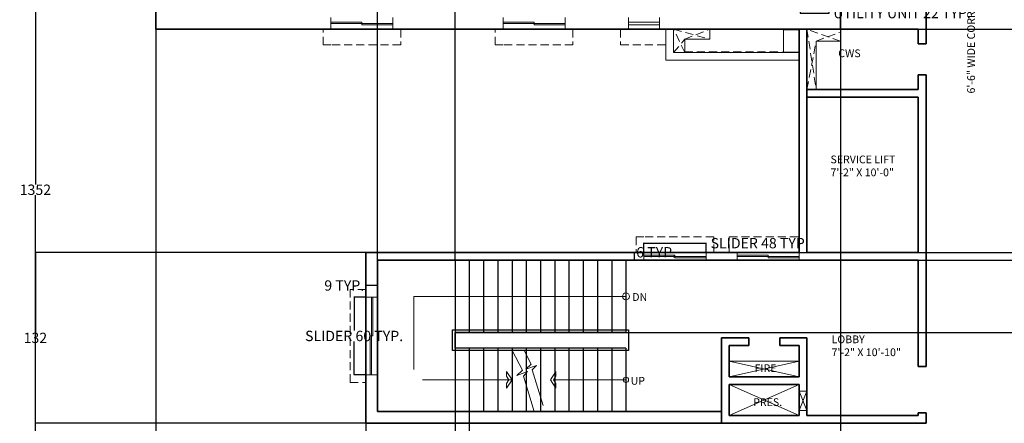
# Model space of a CAD drawing. Units: inches. Extents: x 3343 to 4790, y 1140 to 2641.
# Tile 2 of 10: x 3343 to 4104, y 1710 to 2022. Entities that reach past the tile are written whole.
import ezdxf

# ---------------------------------------------------------------- set-up
doc = ezdxf.new("R2010")
doc.units = ezdxf.units.IN
doc.header["$LTSCALE"] = 5
doc.header["$MEASUREMENT"] = 0
doc.linetypes.add('HIDDEN', pattern=[0.375, 0.25, -0.125])
for name, color, linetype, lineweight in [('A-ANNO-DIMS', 2, 'Continuous', 18), ('A-ANNO-SYMB', 7, 'Continuous', 18), ('A-ANNO-TEXT', 7, 'Continuous', 18), ('A-AREA-IDEN', 7, 'Continuous', 18), ('A-FLOR-HIDN', 8, 'HIDDEN', 13), ('A-FLOR-SHFT', 8, 'Continuous', 18), ('A-FLOR-STRS', 7, 'Continuous', 25), ('A-GLAZ', 4, 'Continuous', 18), ('A-WALL', 7, 'Continuous', 35)]:
    doc.layers.add(name, color=color, linetype=linetype, lineweight=lineweight)
doc.styles.get("Standard").update_dxf_attribs({"font": 'arial.ttf'})
doc.dimstyles.get("Standard").update_dxf_attribs({"dimtxt": 8, "dimasz": 0.18, "dimexe": 0.18, "dimexo": 0.0625, "dimgap": 0.09, "dimtad": 0, "dimtih": 1, "dimtoh": 1, "dimdec": 1, "dimzin": 0, "dimdsep": 46, "dimlunit": 3, "dimtxsty": 'Standard', "dimcen": 0.09, "dimadec": 0, "dimazin": 0, "dimtfac": 1, "dimtdec": 1, "dimtofl": 0, "dimtmove": 0, "dimatfit": 3, "dimfxl": 1, "dimtolj": 1, "dimtzin": 0, "dimarcsym": 0})

# ---------------------------------------------------------------- blocks, each defined once
blk = doc.blocks.new('WINDOW-48IN-SLIDING-JAMB9')
for p, q in [((0, 9), (0, 0)), ((48, 9), (48, 0)), ((0, 5.5), (24, 5.5)), ((0, 4.5), (48, 4.5)), ((24, 5.5), (24, 3.5)), ((24, 3.5), (48, 3.5))]:
    blk.add_line(p, q)
blk = doc.blocks.new('WINDOW-24IN-FIXED')
for p, q in [((0, 9), (0, 0)), ((24, 9), (24, 0)), ((0, 5.5), (24, 5.5)), ((0, 3.5), (24, 3.5))]:
    blk.add_line(p, q)
blk = doc.blocks.new('WINDOW-48IN-SLIDING-JAMB6')
at = {"ltscale": 5}
for p, q in [((0, 6), (0, 0)), ((24, 4), (0, 4)), ((48, 3), (0, 3)), ((24, 4), (24, 2)), ((48, 2), (24, 2)), ((48, 6), (48, 0))]:
    blk.add_line(p, q, dxfattribs=at)
blk = doc.blocks.new('WINDOW-60IN-SLIDING')
at = {"ltscale": 5}
for p, q in [((9, 60), (0, 60)), ((4.5, 60), (4.5, 0)), ((5.5, 60), (5.5, 30)), ((5.5, 30), (3.5, 30)), ((3.5, 30), (3.5, 0)), ((9, 0), (0, 0))]:
    blk.add_line(p, q, dxfattribs=at)
blk = doc.blocks.new('*D73')
at = {"layer": 'A-ANNO-DIMS', "color": 0, "lineweight": -2, "ltscale": 5, "transparency": 16777216}
for p, q in [((3945.78, 2029.98), (3945.78, 2026.51)), ((3945.96, 2026.69), (3967.95, 2026.69)), ((3968.13, 2029.98), (3968.13, 2026.51)), ((3968.13, 2026.69), (3968.31, 2026.69))]:
    blk.add_line(p, q, dxfattribs=at)
at = {"layer": 'A-ANNO-DIMS', "color": 0, "ltscale": 5, "transparency": 16777216}
for points in [[(3945.96, 2026.72), (3945.96, 2026.66), (3945.78, 2026.69)], [(3967.95, 2026.72), (3967.95, 2026.66), (3968.13, 2026.69)]]:
    blk.add_solid(points, dxfattribs=at)
at = {"layer": 'Defpoints', "color": 0, "ltscale": 5, "transparency": 16777216}
for p in [(3945.78, 2030.05), (3968.13, 2030.05), (3968.13, 2026.69)]:
    blk.add_point(p, dxfattribs=at)
at = {"layer": 'A-ANNO-DIMS', "color": 0, "ltscale": 5, "transparency": 16777216, "insert": (4024.61, 2026.69), "char_height": 8, "attachment_point": 5}
blk.add_mtext('\\A1;UTILITY UNIT 22 TYP.', dxfattribs=at)
blk = doc.blocks.new('*D77')
at = {"layer": 'A-ANNO-DIMS', "color": 0, "lineweight": -2, "ltscale": 5, "transparency": 16777216}
for p, q in [((3825.13, 1841.73), (3825.13, 1849.05)), ((3825.31, 1848.87), (3872.95, 1848.87)), ((3873.13, 1841.73), (3873.13, 1849.05)), ((3873.13, 1848.87), (3873.31, 1848.87))]:
    blk.add_line(p, q, dxfattribs=at)
at = {"layer": 'A-ANNO-DIMS', "color": 0, "ltscale": 5, "transparency": 16777216}
for points in [[(3825.31, 1848.9), (3825.31, 1848.84), (3825.13, 1848.87)], [(3872.95, 1848.9), (3872.95, 1848.84), (3873.13, 1848.87)]]:
    blk.add_solid(points, dxfattribs=at)
at = {"layer": 'Defpoints', "color": 0, "ltscale": 5, "transparency": 16777216}
for p in [(3873.13, 1848.87), (3825.13, 1841.67), (3873.13, 1841.67)]:
    blk.add_point(p, dxfattribs=at)
at = {"layer": 'A-ANNO-DIMS', "color": 0, "ltscale": 5, "transparency": 16777216, "insert": (3914.59, 1848.87), "char_height": 8, "attachment_point": 5}
blk.add_mtext('\\A1;SLIDER 48 TYP.', dxfattribs=at)
blk = doc.blocks.new('*D78')
at = {"layer": 'A-ANNO-DIMS', "color": 0, "lineweight": -2, "ltscale": 5, "transparency": 16777216}
for p, q in [((3825.07, 1841.67), (3817.75, 1841.67)), ((3817.93, 1841.67), (3817.93, 1841.85)), ((3817.93, 1841.85), (3818.11, 1841.85)), ((3817.93, 1835.85), (3817.93, 1841.49)), ((3825.07, 1835.67), (3817.75, 1835.67))]:
    blk.add_line(p, q, dxfattribs=at)
at = {"layer": 'A-ANNO-DIMS', "color": 0, "ltscale": 5, "transparency": 16777216}
for points in [[(3817.9, 1841.49), (3817.96, 1841.49), (3817.93, 1841.67)], [(3817.9, 1835.85), (3817.96, 1835.85), (3817.93, 1835.67)]]:
    blk.add_solid(points, dxfattribs=at)
at = {"layer": 'Defpoints', "color": 0, "ltscale": 5, "transparency": 16777216}
for p in [(3817.93, 1841.67), (3825.13, 1841.67), (3825.13, 1835.67)]:
    blk.add_point(p, dxfattribs=at)
at = {"layer": 'A-ANNO-DIMS', "color": 0, "ltscale": 5, "transparency": 16777216, "insert": (3834.58, 1841.85), "char_height": 8, "attachment_point": 5}
blk.add_mtext('\\A1;6 TYP.', dxfattribs=at)
blk = doc.blocks.new('*D79')
at = {"layer": 'A-ANNO-DIMS', "color": 0, "lineweight": -2, "ltscale": 5, "transparency": 16777216}
for p, q in [((3610.19, 1807.17), (3601.07, 1807.17)), ((3601.25, 1806.99), (3601.25, 1781.4)), ((3601.25, 1747.35), (3601.25, 1772.94)), ((3610.19, 1747.17), (3601.07, 1747.17))]:
    blk.add_line(p, q, dxfattribs=at)
at = {"layer": 'A-ANNO-DIMS', "color": 0, "ltscale": 5, "transparency": 16777216}
for points in [[(3601.22, 1806.99), (3601.28, 1806.99), (3601.25, 1807.17)], [(3601.22, 1747.35), (3601.28, 1747.35), (3601.25, 1747.17)]]:
    blk.add_solid(points, dxfattribs=at)
at = {"layer": 'Defpoints', "color": 0, "ltscale": 5, "transparency": 16777216}
for p in [(3610.25, 1807.17), (3601.25, 1747.17), (3610.25, 1747.17)]:
    blk.add_point(p, dxfattribs=at)
at = {"layer": 'A-ANNO-DIMS', "color": 0, "ltscale": 5, "transparency": 16777216, "insert": (3601.25, 1777.17), "char_height": 8, "attachment_point": 5}
blk.add_mtext('\\A1;SLIDER 60 TYP.', dxfattribs=at)
blk = doc.blocks.new('*D80')
at = {"layer": 'A-ANNO-DIMS', "color": 0, "lineweight": -2, "ltscale": 5, "transparency": 16777216}
for p, q in [((3610.25, 1816.17), (3610.07, 1816.17)), ((3610.25, 1807.23), (3610.25, 1816.35)), ((3619.07, 1816.17), (3610.43, 1816.17)), ((3619.25, 1807.23), (3619.25, 1816.35))]:
    blk.add_line(p, q, dxfattribs=at)
at = {"layer": 'A-ANNO-DIMS', "color": 0, "ltscale": 5, "transparency": 16777216}
for points in [[(3610.43, 1816.2), (3610.43, 1816.14), (3610.25, 1816.17)], [(3619.07, 1816.2), (3619.07, 1816.14), (3619.25, 1816.17)]]:
    blk.add_solid(points, dxfattribs=at)
at = {"layer": 'Defpoints', "color": 0, "ltscale": 5, "transparency": 16777216}
for p in [(3610.25, 1816.17), (3610.25, 1807.17), (3619.25, 1807.17)]:
    blk.add_point(p, dxfattribs=at)
at = {"layer": 'A-ANNO-DIMS', "color": 0, "ltscale": 5, "transparency": 16777216, "insert": (3593.62, 1816.17), "char_height": 8, "attachment_point": 5}
blk.add_mtext('\\A1;9 TYP.', dxfattribs=at)
blk = doc.blocks.new('*D84')
at = {"layer": 'A-ANNO-DIMS', "color": 0, "lineweight": -2, "ltscale": 5, "transparency": 16777216}
for p, q in [((3448.07, 2566.16), (3354.8, 2566.16)), ((3354.98, 2565.98), (3354.98, 1894.31)), ((3354.98, 1214.29), (3354.98, 1885.96)), ((4015.58, 1214.11), (3354.8, 1214.11))]:
    blk.add_line(p, q, dxfattribs=at)
at = {"layer": 'A-ANNO-DIMS', "color": 0, "ltscale": 5, "transparency": 16777216}
for points in [[(3354.95, 2565.98), (3355.01, 2565.98), (3354.98, 2566.16)], [(3354.95, 1214.29), (3355.01, 1214.29), (3354.98, 1214.11)]]:
    blk.add_solid(points, dxfattribs=at)
at = {"layer": 'Defpoints', "color": 0, "ltscale": 5, "transparency": 16777216}
for p in [(3448.13, 2566.16), (3354.98, 1214.11), (4015.65, 1214.11)]:
    blk.add_point(p, dxfattribs=at)
at = {"layer": 'A-ANNO-DIMS', "color": 0, "ltscale": 5, "transparency": 16777216, "insert": (3354.98, 1890.14), "char_height": 8, "attachment_point": 5}
blk.add_mtext('\\A1;1352', dxfattribs=at)
blk = doc.blocks.new('*D85')
at = {"layer": 'A-ANNO-DIMS', "color": 0, "lineweight": -2, "ltscale": 5, "transparency": 16777216}
for p, q in [((3448.13, 2014.1), (3448.13, 1144.78)), ((3977.13, 2014.1), (3977.13, 1144.78)), ((3448.31, 1144.96), (3703.69, 1144.96)), ((3976.95, 1144.96), (3721.57, 1144.96))]:
    blk.add_line(p, q, dxfattribs=at)
at = {"layer": 'A-ANNO-DIMS', "color": 0, "ltscale": 5, "transparency": 16777216}
for points in [[(3448.31, 1144.99), (3448.31, 1144.93), (3448.13, 1144.96)], [(3976.95, 1144.99), (3976.95, 1144.93), (3977.13, 1144.96)]]:
    blk.add_solid(points, dxfattribs=at)
at = {"layer": 'Defpoints', "color": 0, "ltscale": 5, "transparency": 16777216}
for p in [(3448.13, 2014.16), (3977.13, 2014.16), (3977.13, 1144.96)]:
    blk.add_point(p, dxfattribs=at)
at = {"layer": 'A-ANNO-DIMS', "color": 0, "ltscale": 5, "transparency": 16777216, "insert": (3712.63, 1144.96), "char_height": 8, "attachment_point": 5}
blk.add_mtext('\\A1;529', dxfattribs=at)
blk = doc.blocks.new('*D87')
at = {"layer": 'A-ANNO-DIMS', "color": 0, "lineweight": -2, "ltscale": 5, "transparency": 16777216}
for p, q in [((3977.19, 2566.16), (4773.46, 2566.16)), ((4773.28, 2565.98), (4773.28, 2294.34)), ((4773.28, 2014.34), (4773.28, 2285.99)), ((3977.19, 2014.16), (4773.46, 2014.16))]:
    blk.add_line(p, q, dxfattribs=at)
at = {"layer": 'A-ANNO-DIMS', "color": 0, "ltscale": 5, "transparency": 16777216}
for points in [[(4773.25, 2565.98), (4773.31, 2565.98), (4773.28, 2566.16)], [(4773.25, 2014.34), (4773.31, 2014.34), (4773.28, 2014.16)]]:
    blk.add_solid(points, dxfattribs=at)
at = {"layer": 'Defpoints', "color": 0, "ltscale": 5, "transparency": 16777216}
for p in [(3977.13, 2566.16), (3977.13, 2014.16), (4773.28, 2014.16)]:
    blk.add_point(p, dxfattribs=at)
at = {"layer": 'A-ANNO-DIMS', "color": 0, "ltscale": 5, "transparency": 16777216, "insert": (4773.28, 2290.16), "char_height": 8, "attachment_point": 5}
blk.add_mtext('\\A1;552', dxfattribs=at)
blk = doc.blocks.new('*D90')
at = {"layer": 'A-ANNO-DIMS', "color": 0, "lineweight": -2, "ltscale": 5, "transparency": 16777216}
for p, q in [((3610.19, 1841.67), (3354.8, 1841.67)), ((3354.98, 1841.49), (3354.98, 1779.85)), ((3354.98, 1709.85), (3354.98, 1771.49)), ((3610.19, 1709.67), (3354.8, 1709.67))]:
    blk.add_line(p, q, dxfattribs=at)
at = {"layer": 'A-ANNO-DIMS', "color": 0, "ltscale": 5, "transparency": 16777216}
for points in [[(3354.95, 1841.49), (3355.01, 1841.49), (3354.98, 1841.67)], [(3354.95, 1709.85), (3355.01, 1709.85), (3354.98, 1709.67)]]:
    blk.add_solid(points, dxfattribs=at)
at = {"layer": 'Defpoints', "color": 0, "ltscale": 5, "transparency": 16777216}
for p in [(3354.98, 1841.67), (3610.25, 1841.67), (3610.25, 1709.67)]:
    blk.add_point(p, dxfattribs=at)
at = {"layer": 'A-ANNO-DIMS', "color": 0, "ltscale": 5, "transparency": 16777216, "insert": (3354.98, 1775.67), "char_height": 8, "attachment_point": 5}
blk.add_mtext('\\A1;132', dxfattribs=at)
blk = doc.blocks.new('*D94')
at = {"layer": 'A-ANNO-DIMS', "color": 0, "lineweight": -2, "ltscale": 5, "transparency": 16777216}
for p, q in [((3448.13, 2014.1), (3448.13, 1144.78)), ((3610.25, 1841.61), (3610.25, 1144.78)), ((3448.31, 1144.96), (3512.91, 1144.96)), ((3610.07, 1144.96), (3545.47, 1144.96))]:
    blk.add_line(p, q, dxfattribs=at)
at = {"layer": 'A-ANNO-DIMS', "color": 0, "ltscale": 5, "transparency": 16777216}
for points in [[(3448.31, 1144.99), (3448.31, 1144.93), (3448.13, 1144.96)], [(3610.07, 1144.99), (3610.07, 1144.93), (3610.25, 1144.96)]]:
    blk.add_solid(points, dxfattribs=at)
at = {"layer": 'Defpoints', "color": 0, "ltscale": 5, "transparency": 16777216}
for p in [(3448.13, 2014.16), (3610.25, 1841.67), (3610.25, 1144.96)]:
    blk.add_point(p, dxfattribs=at)
at = {"layer": 'A-ANNO-DIMS', "color": 0, "ltscale": 5, "transparency": 16777216, "insert": (3529.19, 1144.96), "char_height": 8, "attachment_point": 5}
blk.add_mtext('\\A1;162.12', dxfattribs=at)
blk = doc.blocks.new('*D95')
at = {"layer": 'A-ANNO-DIMS', "color": 0, "lineweight": -2, "ltscale": 5, "transparency": 16777216}
for p, q in [((3637.31, 2014.16), (4773.46, 2014.16)), ((4773.28, 2013.98), (4773.28, 1932.09)), ((4773.28, 1841.85), (4773.28, 1923.74)), ((3610.31, 1841.67), (4773.46, 1841.67))]:
    blk.add_line(p, q, dxfattribs=at)
at = {"layer": 'A-ANNO-DIMS', "color": 0, "ltscale": 5, "transparency": 16777216}
for points in [[(4773.25, 2013.98), (4773.31, 2013.98), (4773.28, 2014.16)], [(4773.25, 1841.85), (4773.31, 1841.85), (4773.28, 1841.67)]]:
    blk.add_solid(points, dxfattribs=at)
at = {"layer": 'Defpoints', "color": 0, "ltscale": 5, "transparency": 16777216}
for p in [(3637.25, 2014.16), (3610.25, 1841.67), (4773.28, 1841.67)]:
    blk.add_point(p, dxfattribs=at)
at = {"layer": 'A-ANNO-DIMS', "color": 0, "ltscale": 5, "transparency": 16777216, "insert": (4773.28, 1927.92), "char_height": 8, "attachment_point": 5}
blk.add_mtext('\\A1;172.5', dxfattribs=at)
blk = doc.blocks.new('*D96')
at = {"layer": 'A-ANNO-DIMS', "color": 0, "lineweight": -2, "ltscale": 5, "transparency": 16777216}
for p, q in [((3619.25, 1835.73), (3619.25, 2635.49)), ((3619.43, 2635.31), (3643.42, 2635.31)), ((3679.07, 2635.31), (3655.08, 2635.31)), ((3679.25, 1835.73), (3679.25, 2635.49))]:
    blk.add_line(p, q, dxfattribs=at)
at = {"layer": 'A-ANNO-DIMS', "color": 0, "ltscale": 5, "transparency": 16777216}
for points in [[(3619.43, 2635.34), (3619.43, 2635.28), (3619.25, 2635.31)], [(3679.07, 2635.34), (3679.07, 2635.28), (3679.25, 2635.31)]]:
    blk.add_solid(points, dxfattribs=at)
at = {"layer": 'Defpoints', "color": 0, "ltscale": 5, "transparency": 16777216}
for p in [(3679.25, 2635.31), (3619.25, 1835.67), (3679.25, 1835.67)]:
    blk.add_point(p, dxfattribs=at)
at = {"layer": 'A-ANNO-DIMS', "color": 0, "ltscale": 5, "transparency": 16777216, "insert": (3649.25, 2635.31), "char_height": 8, "attachment_point": 5}
blk.add_mtext('\\A1;60', dxfattribs=at)
blk = doc.blocks.new('*D97')
at = {"layer": 'A-ANNO-DIMS', "color": 0, "lineweight": -2, "ltscale": 5, "transparency": 16777216}
for p, q in [((3679.25, 1718.61), (3679.25, 1144.78)), ((3690.25, 1718.61), (3690.25, 1144.78)), ((3679.43, 1144.96), (3680.08, 1144.96)), ((3690.07, 1144.96), (3689.42, 1144.96))]:
    blk.add_line(p, q, dxfattribs=at)
at = {"layer": 'A-ANNO-DIMS', "color": 0, "ltscale": 5, "transparency": 16777216}
for points in [[(3679.43, 1144.99), (3679.43, 1144.93), (3679.25, 1144.96)], [(3690.07, 1144.99), (3690.07, 1144.93), (3690.25, 1144.96)]]:
    blk.add_solid(points, dxfattribs=at)
at = {"layer": 'Defpoints', "color": 0, "ltscale": 5, "transparency": 16777216}
for p in [(3679.25, 1718.67), (3690.25, 1718.67), (3690.25, 1144.96)]:
    blk.add_point(p, dxfattribs=at)
at = {"layer": 'A-ANNO-DIMS', "color": 0, "ltscale": 5, "transparency": 16777216, "insert": (3684.75, 1144.96), "char_height": 8, "attachment_point": 5}
blk.add_mtext('\\A1;11', dxfattribs=at)
blk = doc.blocks.new('*D98')
at = {"layer": 'A-ANNO-DIMS', "color": 0, "lineweight": -2, "ltscale": 5, "transparency": 16777216}
for p, q in [((3811.31, 1835.67), (4773.46, 1835.67)), ((4773.28, 1835.49), (4773.28, 1811.94)), ((4773.28, 1780.04), (4773.28, 1803.59)), ((3811.31, 1779.86), (4773.46, 1779.86))]:
    blk.add_line(p, q, dxfattribs=at)
at = {"layer": 'A-ANNO-DIMS', "color": 0, "ltscale": 5, "transparency": 16777216}
for points in [[(4773.25, 1835.49), (4773.31, 1835.49), (4773.28, 1835.67)], [(4773.25, 1780.04), (4773.31, 1780.04), (4773.28, 1779.86)]]:
    blk.add_solid(points, dxfattribs=at)
at = {"layer": 'Defpoints', "color": 0, "ltscale": 5, "transparency": 16777216}
for p in [(3811.25, 1835.67), (3811.25, 1779.86), (4773.28, 1779.86)]:
    blk.add_point(p, dxfattribs=at)
at = {"layer": 'A-ANNO-DIMS', "color": 0, "ltscale": 5, "transparency": 16777216, "insert": (4773.28, 1807.76), "char_height": 8, "attachment_point": 5}
blk.add_mtext('\\A1;55.81', dxfattribs=at)

msp = doc.modelspace()

# ---------------------------------------------------------------- linework, layer by layer
at = {"layer": 'A-ANNO-SYMB', "ltscale": 5}
for p, q in [((3811.248, 1807.763), (3647.424, 1807.763)), ((3647.424, 1807.763), (3647.424, 1751.228)), ((3723.248, 1765.857), (3731.265, 1750.62)), ((3732.699, 1765.857), (3738.168, 1755.46)), ((3723.248, 1743.263), (3719.017, 1749.732)), ((3719.017, 1749.732), (3719.017, 1746.086)), ((3731.265, 1750.62), (3727.024, 1746.671)), ((3738.168, 1755.46), (3733.927, 1751.512)), ((3733.927, 1751.512), (3742.238, 1754.464)), ((3742.238, 1754.464), (3738.938, 1750.901)), ((3738.938, 1750.901), (3747.392, 1723.51)), ((3752.885, 1743.263), (3757.116, 1749.732)), ((3757.116, 1749.732), (3757.116, 1746.086)), ((3690.248, 1743.263), (3654.175, 1743.263)), ((3690.248, 1743.263), (3723.248, 1743.263)), ((3719.017, 1746.086), (3720.752, 1743.263)), ((3723.248, 1743.263), (3719.017, 1736.794)), ((3719.017, 1740.441), (3720.752, 1743.263)), ((3727.024, 1746.671), (3735.334, 1749.624)), ((3735.334, 1749.624), (3732.034, 1746.061)), ((3732.034, 1746.061), (3740.489, 1718.669)), ((3752.885, 1743.263), (3757.116, 1736.794)), ((3757.116, 1746.086), (3755.381, 1743.263)), ((3757.116, 1740.441), (3755.381, 1743.263)), ((3756.248, 1743.263), (3811.248, 1743.263)), ((3719.017, 1736.794), (3719.017, 1740.441)), ((3757.116, 1736.794), (3757.116, 1740.441))]:
    msp.add_line(p, q, dxfattribs=at)
for centre, radius in [((3811.248, 1807.763), 2.654), ((3811.248, 1743.263), 2.078)]:
    msp.add_circle(centre, radius, dxfattribs=at)
at = {"layer": 'A-FLOR-HIDN', "ltscale": 5}
for p, q in [((3577.248, 2002.161), (3577.248, 2014.161)), ((3631.248, 2014.161), (3637.248, 2014.161)), ((3637.248, 2014.161), (3637.248, 2002.161)), ((3710.353, 2002.161), (3710.353, 2014.161)), ((3764.353, 2014.161), (3770.353, 2014.161)), ((3770.353, 2014.161), (3770.353, 2002.161)), ((3813.16, 2014.161), (3807.16, 2014.161)), ((3807.16, 2014.161), (3807.16, 2002.161)), ((3856.673, 1996.161), (3848.13, 2014.161)), ((3848.13, 2014.161), (3876.122, 2006.459)), ((3856.673, 2006.459), (3876.122, 2014.161)), ((3977.13, 2005.073), (3951.13, 2014.161)), ((3951.13, 2014.161), (3958.254, 1967.669)), ((3958.254, 2005.073), (3977.13, 2012.008)), ((3583.248, 2002.161), (3577.248, 2002.161)), ((3637.248, 2002.161), (3583.248, 2002.161)), ((3716.353, 2002.161), (3710.353, 2002.161)), ((3770.353, 2002.161), (3716.353, 2002.161)), ((3807.16, 2002.161), (3842.13, 2002.161)), ((3848.13, 1996.161), (3856.673, 2006.459)), ((3951.13, 1967.669), (3958.254, 2005.073)), ((3856.673, 1996.696), (3940.654, 1996.58)), ((3825.13, 1853.669), (3819.13, 1853.669)), ((3819.13, 1853.669), (3819.13, 1841.669)), ((3879.13, 1853.669), (3825.13, 1853.669)), ((3879.13, 1841.669), (3879.13, 1853.669)), ((3891.13, 1841.669), (3891.13, 1853.669)), ((3891.13, 1853.669), (3945.13, 1853.669)), ((3873.13, 1841.669), (3879.13, 1841.669)), ((3897.13, 1841.669), (3891.13, 1841.669)), ((3610.248, 1813.169), (3598.248, 1813.169)), ((3598.248, 1813.169), (3598.248, 1747.169)), ((3610.248, 1807.169), (3610.248, 1813.169)), ((3598.248, 1747.169), (3598.248, 1741.169)), ((3598.248, 1741.169), (3610.248, 1741.169))]:
    msp.add_line(p, q, dxfattribs=at)
at = {"layer": 'A-FLOR-SHFT', "ltscale": 5}
for p, q in [((3842.13, 2014.161), (3842.13, 1990.161)), ((3876.122, 2014.161), (3876.122, 2006.459)), ((3951.13, 1991.472), (3951.13, 2014.161)), ((3977.13, 2014.161), (3977.13, 2005.073)), ((3876.122, 2006.459), (3856.673, 2006.459)), ((3856.673, 2006.459), (3856.673, 1996.161)), ((3977.13, 2005.073), (3958.254, 2005.073)), ((3958.254, 2005.073), (3958.254, 1967.669)), ((3842.13, 1990.161), (3945.13, 1990.161)), ((3891.13, 1757.669), (3945.13, 1757.669)), ((3945.13, 1757.669), (3891.13, 1745.669)), ((3891.13, 1757.669), (3945.13, 1745.669)), ((3891.13, 1739.669), (3945.13, 1715.669)), ((3945.13, 1739.669), (3891.13, 1715.669)), ((3945.13, 1734.618), (3951.13, 1719.611)), ((3945.13, 1719.611), (3951.13, 1734.618))]:
    msp.add_line(p, q, dxfattribs=at)
msp.add_lwpolyline([(3848.13, 2014.161), (3848.13, 1996.161), (3945.13, 1996.161), (3945.13, 2014.161)], dxfattribs=at)
for points in [[(3945.13, 2013.712), (3933.112, 2013.712), (3933.112, 1996.58), (3945.13, 1996.58)], [(3945.13, 1734.618), (3951.13, 1734.618), (3951.13, 1719.611), (3945.13, 1719.611)]]:
    msp.add_lwpolyline(points, close=True, dxfattribs=at)
at = {"layer": 'A-FLOR-STRS', "ltscale": 5}
for p, q in [((3679.248, 1835.669), (3679.248, 1718.669)), ((3690.248, 1835.669), (3690.248, 1779.857)), ((3701.248, 1835.669), (3701.248, 1779.857)), ((3712.248, 1835.669), (3712.248, 1779.857)), ((3723.248, 1835.669), (3723.248, 1779.857)), ((3734.248, 1835.669), (3734.248, 1779.857)), ((3745.248, 1835.669), (3745.248, 1779.857)), ((3756.248, 1835.669), (3756.248, 1779.857)), ((3767.248, 1835.669), (3767.248, 1779.857)), ((3778.248, 1835.669), (3778.248, 1779.857)), ((3789.248, 1835.669), (3789.248, 1779.857)), ((3800.248, 1835.669), (3800.248, 1779.857)), ((3811.248, 1835.669), (3811.248, 1779.857)), ((3811.248, 1779.857), (3679.248, 1779.857)), ((3811.248, 1767.857), (3679.248, 1767.857)), ((3690.248, 1767.857), (3690.248, 1718.669)), ((3701.248, 1767.857), (3701.248, 1718.669)), ((3712.248, 1767.857), (3712.248, 1718.669)), ((3723.248, 1767.857), (3723.248, 1718.669)), ((3734.248, 1767.857), (3734.248, 1718.669)), ((3745.248, 1767.857), (3745.248, 1718.669)), ((3756.248, 1767.857), (3756.248, 1718.669)), ((3767.248, 1767.857), (3767.248, 1718.669)), ((3778.248, 1767.857), (3778.248, 1718.669)), ((3789.248, 1767.857), (3789.248, 1718.669)), ((3800.248, 1767.857), (3800.248, 1718.669)), ((3811.248, 1767.857), (3811.248, 1718.669))]:
    msp.add_line(p, q, dxfattribs=at)
msp.add_lwpolyline([(3677.248, 1781.857), (3813.248, 1781.857), (3813.248, 1765.857), (3677.248, 1765.857)], close=True, dxfattribs=at)
msp.add_lwpolyline([(3811.248, 1767.857), (3679.248, 1767.857), (3679.248, 1779.857), (3811.248, 1779.857)], dxfattribs=at)
at = {"layer": 'A-WALL'}
for p, q in [((3448.13, 2566.161), (3448.13, 2014.161)), ((3977.13, 2302.46), (3977.13, 2014.161)), ((4043.13, 2045.194), (4043.13, 2002.915)), ((3945.13, 2014.161), (3945.13, 1841.669)), ((3951.13, 2014.161), (3951.13, 1841.669)), ((4037.13, 2014.161), (4037.13, 2002.915)), ((4037.13, 1978.915), (4037.13, 1967.669)), ((4043.13, 1978.915), (4043.13, 1835.669)), ((4037.13, 1961.669), (4037.13, 1841.669))]:
    msp.add_line(p, q, dxfattribs=at)
at = {"layer": 'A-WALL', "ltscale": 5}
for p, q in [((3977.13, 2014.161), (3448.13, 2014.161)), ((3945.13, 1961.669), (3945.13, 2014.161)), ((3951.13, 1967.669), (3951.13, 2014.161)), ((3977.13, 2014.161), (4037.13, 2014.161)), ((4037.13, 2002.915), (4043.13, 2002.915)), ((4037.13, 1978.915), (4043.13, 1978.915)), ((4037.13, 1967.669), (3951.13, 1967.669)), ((4037.13, 1961.669), (3951.13, 1961.669)), ((3945.13, 1841.669), (3610.248, 1841.669)), ((3610.248, 1841.669), (3610.248, 1709.669)), ((4037.13, 1841.669), (3951.13, 1841.669)), ((3951.13, 1835.669), (3619.248, 1835.669)), ((3619.248, 1835.669), (3619.248, 1718.669)), ((4037.13, 1835.669), (3951.13, 1835.669)), ((4037.13, 1835.669), (4037.13, 1753.669)), ((4043.13, 1839.035), (4043.13, 1753.669)), ((3885.13, 1775.669), (3885.13, 1709.669)), ((3906.13, 1775.669), (3885.13, 1775.669)), ((3906.13, 1769.669), (3906.13, 1775.669)), ((3951.13, 1775.669), (3930.13, 1775.669)), ((3930.13, 1769.669), (3930.13, 1775.669)), ((3951.13, 1775.669), (3951.13, 1715.669)), ((3891.13, 1769.669), (3891.13, 1745.669)), ((3906.13, 1769.669), (3891.13, 1769.669)), ((3945.13, 1769.669), (3930.13, 1769.669)), ((3945.13, 1769.669), (3945.13, 1745.669)), ((4037.13, 1753.669), (4043.13, 1753.669)), ((3945.13, 1745.669), (3891.13, 1745.669)), ((3945.13, 1739.669), (3891.13, 1739.669)), ((3891.13, 1739.669), (3891.13, 1715.669)), ((3945.13, 1739.669), (3945.13, 1715.669)), ((3885.13, 1718.669), (3619.248, 1718.669)), ((3945.13, 1715.669), (3891.13, 1715.669)), ((4037.13, 1715.669), (3951.13, 1715.669)), ((4037.13, 1717.669), (4043.13, 1717.669)), ((4037.13, 1717.669), (4037.13, 1715.669)), ((4043.13, 1717.669), (4043.13, 1709.669)), ((3885.13, 1709.669), (3610.248, 1709.669)), ((4043.13, 1709.669), (3885.13, 1709.669))]:
    msp.add_line(p, q, dxfattribs=at)

# ---------------------------------------------------------------- block references
at = {"layer": 'A-GLAZ'}
for name, p in [('WINDOW-48IN-SLIDING-JAMB9', (3583.248, 2014.161)), ('WINDOW-48IN-SLIDING-JAMB9', (3716.353, 2014.161)), ('WINDOW-48IN-SLIDING-JAMB6', (3825.13, 1835.669)), ('WINDOW-48IN-SLIDING-JAMB6', (3897.13, 1835.669))]:
    msp.add_blockref(name, p, dxfattribs=at)
at = {"layer": 'A-GLAZ', "rotation": 180}
for name, p in [('WINDOW-24IN-FIXED', (3837.159, 2023.161)), ('WINDOW-60IN-SLIDING', (3619.248, 1807.169))]:
    msp.add_blockref(name, p, dxfattribs=at)

# ---------------------------------------------------------------- texts
at = {"layer": 'A-ANNO-TEXT', "ltscale": 5, "char_height": 6, "attachment_point": 1}
for s, insert in [('DN', (3816.147, 1810.265)), ('UP', (3814.923, 1745.499))]:
    msp.add_mtext_dynamic_manual_height_columns(s, width=189.69543, gutter_width=1, heights=[0], dxfattribs=dict(at, insert=insert))
at = {"layer": 'A-AREA-IDEN', "ltscale": 5, "insert": (4074.933, 1964.53), "char_height": 6, "attachment_point": 1, "rotation": 90}
msp.add_mtext_dynamic_manual_height_columns('6\'-6" WIDE CORRIDIR', width=189.69543, gutter_width=1, heights=[0], dxfattribs=at)
at = {"layer": 'A-AREA-IDEN', "ltscale": 5, "char_height": 6, "attachment_point": 1}
for s, insert in [('CWS', (3975.322, 1998.599)), ('SERVICE LIFT\\P7\'-2" X 10\'-0"', (3969.304, 1916.586)), ('LOBBY\\P7\'-2" X 10\'-10"', (3970.163, 1777.562)), ('FIRE', (3910.599, 1755.227)), ('PRES.', (3909.632, 1729.003))]:
    msp.add_mtext_dynamic_manual_height_columns(s, width=189.69543, gutter_width=1, heights=[0], dxfattribs=dict(at, insert=insert))

# ---------------------------------------------------------------- dimensions: what is measured, and where the dimension line sits
at = {"layer": 'A-ANNO-DIMS', "ltscale": 5}
for base, p1, p2, override, picture, middle in [((3679.248, 2635.311), (3619.248, 1835.669), (3679.248, 1835.669), {"dimdec": 0, "dimlfac": 1, "dimrnd": 0, "dimzin": 0, "dimdsep": 46, "dimlunit": 2}, '*D96', (3649.248, 2635.311)), ((3977.13, 1144.962), (3448.13, 2014.161), (3977.13, 2014.161), {"dimdec": 0, "dimlfac": 1, "dimrnd": 0, "dimzin": 0, "dimdsep": 46, "dimlunit": 2}, '*D85', (3712.63, 1144.962)), ((3610.248, 1144.962), (3448.13, 2014.161), (3610.248, 1841.669), {"dimdec": 2, "dimlfac": 1, "dimrnd": 0, "dimzin": 0, "dimdsep": 46, "dimlunit": 2}, '*D94', (3529.189, 1144.962)), ((3690.248, 1144.962), (3679.248, 1718.669), (3690.248, 1718.669), {"dimdec": 0, "dimlfac": 1, "dimrnd": 0, "dimzin": 0, "dimdsep": 46, "dimlunit": 2}, '*D97', (3684.748, 1144.962))]:
    dim = msp.add_linear_dim(base=base, p1=p1, p2=p2, dimstyle='Standard', override=override, dxfattribs=at)
    dim.commit()
    dim.dimension.update_dxf_attribs({"geometry": picture, "text_midpoint": middle})
for base, p1, p2, override, picture, middle in [((3354.98, 1214.112), (3448.13, 2566.161), (4015.647, 1214.112), {"dimdec": 0, "dimlfac": 1, "dimrnd": 0, "dimzin": 0, "dimdsep": 46, "dimlunit": 2}, '*D84', (3354.98, 1890.137)), ((4773.28, 2014.161), (3977.13, 2566.161), (3977.13, 2014.161), {"dimdec": 0, "dimlfac": 1, "dimrnd": 0, "dimzin": 0, "dimdsep": 46, "dimlunit": 2}, '*D87', (4773.28, 2290.161)), ((4773.28, 1841.669), (3637.248, 2014.161), (3610.248, 1841.669), {"dimdec": 1, "dimlfac": 1, "dimrnd": 0, "dimzin": 0, "dimdsep": 46, "dimlunit": 2}, '*D95', (4773.28, 1927.915)), ((3354.98, 1841.669), (3610.248, 1709.669), (3610.248, 1841.669), {"dimdec": 0, "dimlfac": 1, "dimrnd": 0, "dimzin": 0, "dimdsep": 46, "dimlunit": 2}, '*D90', (3354.98, 1775.669)), ((4773.28, 1779.857), (3811.248, 1835.669), (3811.248, 1779.857), {"dimdec": 2, "dimlfac": 1, "dimrnd": 0, "dimzin": 0, "dimdsep": 46, "dimlunit": 2}, '*D98', (4773.28, 1807.763))]:
    dim = msp.add_linear_dim(base=base, p1=p1, p2=p2, angle=90, dimstyle='Standard', override=override, dxfattribs=at)
    dim.commit()
    dim.dimension.update_dxf_attribs({"geometry": picture, "text_midpoint": middle})
for base, p1, p2, text, picture, middle in [((3968.13, 2026.694), (3945.775, 2030.047), (3968.13, 2030.047), 'UTILITY UNIT <> TYP.', '*D73', (4024.607, 2026.694)), ((3873.13, 1848.869), (3825.13, 1841.669), (3873.13, 1841.669), 'SLIDER <> TYP.', '*D77', (3914.589, 1848.869))]:
    dim = msp.add_linear_dim(base=base, p1=p1, p2=p2, text=text, dimstyle='Standard', override={"dimdec": 0, "dimlfac": 1, "dimrnd": 0, "dimzin": 0, "dimdsep": 46, "dimlunit": 2}, dxfattribs=at)
    dim.commit()
    dim.dimension.update_dxf_attribs({"geometry": picture, "text_midpoint": middle})
for base, p1, p2, angle, text, picture, middle in [((3817.93, 1841.669), (3825.13, 1835.669), (3825.13, 1841.669), 90, '<> TYP.', '*D78', (3834.584, 1841.849)), ((3610.248, 1816.169), (3619.248, 1807.169), (3610.248, 1807.169), 180, '<> TYP.', '*D80', (3593.615, 1816.169)), ((3601.248, 1747.169), (3610.248, 1807.169), (3610.248, 1747.169), 270, 'SLIDER <> TYP.', '*D79', (3601.248, 1777.169))]:
    dim = msp.add_linear_dim(base=base, p1=p1, p2=p2, angle=angle, text=text, dimstyle='Standard', override={"dimdec": 0, "dimlfac": 1, "dimrnd": 0, "dimzin": 0, "dimdsep": 46, "dimlunit": 2}, dxfattribs=at)
    dim.commit()
    dim.dimension.update_dxf_attribs({"geometry": picture, "text_midpoint": middle})

doc.saveas('drawing.dxf')
